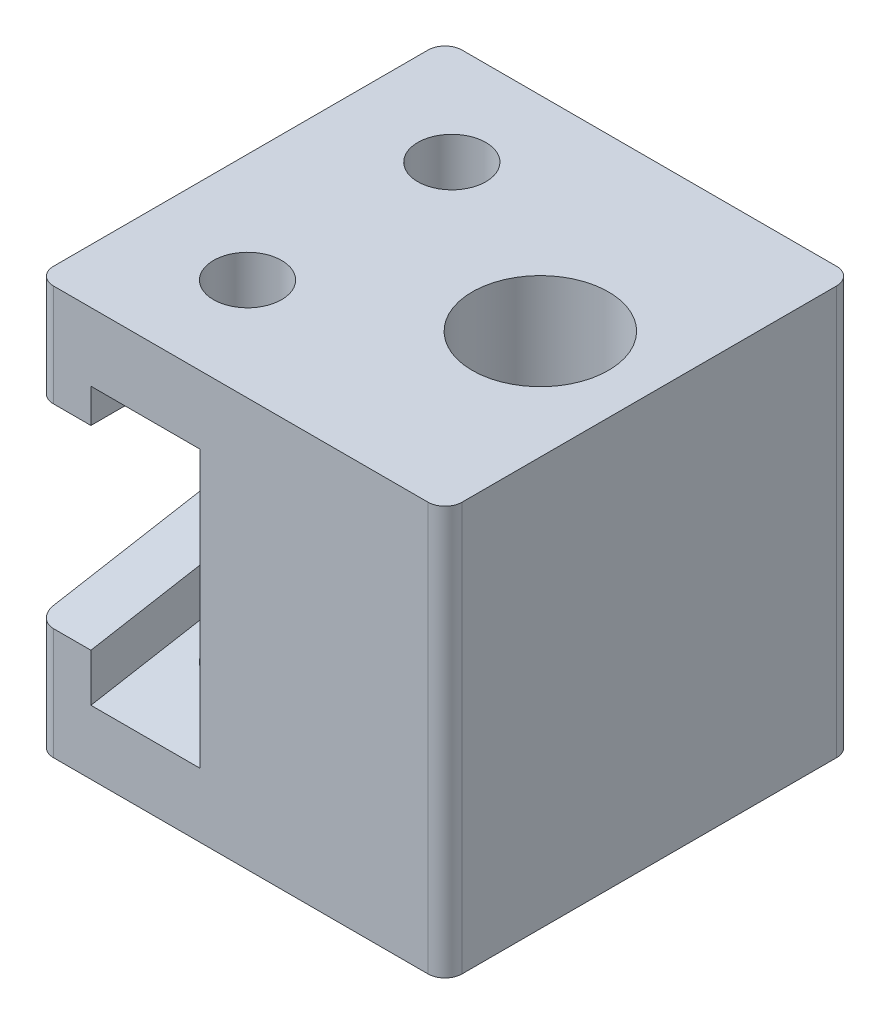
ISO-10303-21;
HEADER;
FILE_DESCRIPTION(('STEP AP214'),'2;1');
FILE_NAME('part.step','',(''),(''),'','','');
FILE_SCHEMA(('AUTOMOTIVE_DESIGN { 1 0 10303 214 1 1 1 1 }'));
ENDSEC;
DATA;
#1=APPLICATION_CONTEXT('core data for automotive mechanical design processes');
#2=APPLICATION_PROTOCOL_DEFINITION('international standard','automotive_design',2000,#1);
#3=PRODUCT_CONTEXT('',#1,'mechanical');
#4=PRODUCT('Part','Part','',(#3));
#5=PRODUCT_RELATED_PRODUCT_CATEGORY('part','',(#4));
#6=PRODUCT_DEFINITION_FORMATION('','',#4);
#7=PRODUCT_DEFINITION_CONTEXT('part definition',#1,'design');
#8=PRODUCT_DEFINITION('design','',#6,#7);
#9=PRODUCT_DEFINITION_SHAPE('','',#8);
#10=(LENGTH_UNIT() NAMED_UNIT(*) SI_UNIT(.MILLI.,.METRE.));
#11=(NAMED_UNIT(*) PLANE_ANGLE_UNIT() SI_UNIT($,.RADIAN.));
#12=(NAMED_UNIT(*) SI_UNIT($,.STERADIAN.) SOLID_ANGLE_UNIT());
#13=UNCERTAINTY_MEASURE_WITH_UNIT(LENGTH_MEASURE(1.E-05),#10,'distance_accuracy_value','');
#14=(GEOMETRIC_REPRESENTATION_CONTEXT(3) GLOBAL_UNCERTAINTY_ASSIGNED_CONTEXT((#13)) GLOBAL_UNIT_ASSIGNED_CONTEXT((#10,
#11,#12)) REPRESENTATION_CONTEXT('',''));
#15=CARTESIAN_POINT('',(0.,0.,0.));
#16=DIRECTION('',(0.,0.,1.));
#17=DIRECTION('',(1.,0.,0.));
#18=AXIS2_PLACEMENT_3D('',#15,#16,#17);
#19=CARTESIAN_POINT('',(0.,0.,38.1));
#20=DIRECTION('',(0.,0.,-1.));
#21=DIRECTION('',(-1.,0.,0.));
#22=AXIS2_PLACEMENT_3D('',#19,#20,#21);
#23=PLANE('',#22);
#24=DIRECTION('',(1.,0.,0.));
#25=VECTOR('',#24,1.);
#26=CARTESIAN_POINT('',(-38.1,-38.1,38.1));
#27=LINE('',#26,#25);
#28=CARTESIAN_POINT('',(-34.925,-38.1,38.1));
#29=VERTEX_POINT('',#28);
#30=CARTESIAN_POINT('',(34.925,-38.1,38.1));
#31=VERTEX_POINT('',#30);
#32=EDGE_CURVE('E229',#29,#31,#27,.T.);
#33=ORIENTED_EDGE('',*,*,#32,.T.);
#34=DIRECTION('',(0.,1.,0.));
#35=VECTOR('',#34,1.);
#36=CARTESIAN_POINT('',(34.925,0.,38.1));
#37=LINE('',#36,#35);
#38=CARTESIAN_POINT('',(34.925,38.1,38.1));
#39=VERTEX_POINT('',#38);
#40=EDGE_CURVE('E11',#31,#39,#37,.T.);
#41=ORIENTED_EDGE('',*,*,#40,.T.);
#42=DIRECTION('',(-1.,0.,0.));
#43=VECTOR('',#42,1.);
#44=CARTESIAN_POINT('',(-38.1,38.1,38.1));
#45=LINE('',#44,#43);
#46=CARTESIAN_POINT('',(-34.925,38.1,38.1));
#47=VERTEX_POINT('',#46);
#48=EDGE_CURVE('E223',#39,#47,#45,.T.);
#49=ORIENTED_EDGE('',*,*,#48,.T.);
#50=DIRECTION('',(0.,-1.,0.));
#51=VECTOR('',#50,1.);
#52=CARTESIAN_POINT('',(-34.925,0.,38.1));
#53=LINE('',#52,#51);
#54=CARTESIAN_POINT('',(-34.925,19.05,38.1));
#55=VERTEX_POINT('',#54);
#56=EDGE_CURVE('E289',#47,#55,#53,.T.);
#57=ORIENTED_EDGE('',*,*,#56,.T.);
#58=DIRECTION('',(-1.,0.,0.));
#59=VECTOR('',#58,1.);
#60=CARTESIAN_POINT('',(-27.94,19.05,38.1));
#61=LINE('',#60,#59);
#62=CARTESIAN_POINT('',(-27.94,19.05,38.1));
#63=VERTEX_POINT('',#62);
#64=EDGE_CURVE('E206',#63,#55,#61,.T.);
#65=ORIENTED_EDGE('',*,*,#64,.F.);
#66=DIRECTION('',(0.,1.,0.));
#67=VECTOR('',#66,1.);
#68=CARTESIAN_POINT('',(-27.94,25.4,38.1));
#69=LINE('',#68,#67);
#70=CARTESIAN_POINT('',(-27.94,25.4,38.1));
#71=VERTEX_POINT('',#70);
#72=EDGE_CURVE('E325',#63,#71,#69,.T.);
#73=ORIENTED_EDGE('',*,*,#72,.T.);
#74=DIRECTION('',(-1.,0.,0.));
#75=VECTOR('',#74,1.);
#76=CARTESIAN_POINT('',(-7.61999999999999,25.4,38.1));
#77=LINE('',#76,#75);
#78=CARTESIAN_POINT('',(-7.61999999999999,25.4,38.1));
#79=VERTEX_POINT('',#78);
#80=EDGE_CURVE('E198',#79,#71,#77,.T.);
#81=ORIENTED_EDGE('',*,*,#80,.F.);
#82=DIRECTION('',(0.,1.,0.));
#83=VECTOR('',#82,1.);
#84=CARTESIAN_POINT('',(-7.61999999999999,25.4,38.1));
#85=LINE('',#84,#83);
#86=CARTESIAN_POINT('',(-7.61999999999999,-26.1361159299851,38.1));
#87=VERTEX_POINT('',#86);
#88=EDGE_CURVE('E176',#87,#79,#85,.T.);
#89=ORIENTED_EDGE('',*,*,#88,.F.);
#90=DIRECTION('',(-1.,0.,0.));
#91=VECTOR('',#90,1.);
#92=CARTESIAN_POINT('',(-7.61999999999999,-26.1361159299851,38.1));
#93=LINE('',#92,#91);
#94=CARTESIAN_POINT('',(-27.94,-26.1361159299851,38.1));
#95=VERTEX_POINT('',#94);
#96=EDGE_CURVE('E175',#87,#95,#93,.T.);
#97=ORIENTED_EDGE('',*,*,#96,.T.);
#98=CARTESIAN_POINT('',(-27.94,-17.2461159299851,38.1));
#99=VERTEX_POINT('',#98);
#100=EDGE_CURVE('E323',#95,#99,#69,.T.);
#101=ORIENTED_EDGE('',*,*,#100,.T.);
#102=DIRECTION('',(-1.,0.,0.));
#103=VECTOR('',#102,1.);
#104=CARTESIAN_POINT('',(-27.94,-17.2461159299851,38.1));
#105=LINE('',#104,#103);
#106=CARTESIAN_POINT('',(-34.925,-17.2461159299851,38.1));
#107=VERTEX_POINT('',#106);
#108=EDGE_CURVE('E213',#99,#107,#105,.T.);
#109=ORIENTED_EDGE('',*,*,#108,.T.);
#110=DIRECTION('',(0.,-1.,0.));
#111=VECTOR('',#110,1.);
#112=CARTESIAN_POINT('',(-34.925,0.,38.1));
#113=LINE('',#112,#111);
#114=EDGE_CURVE('E48',#107,#29,#113,.T.);
#115=ORIENTED_EDGE('',*,*,#114,.T.);
#116=EDGE_LOOP('',(#33,#41,#49,#57,#65,#73,#81,#89,#97,#101,#109,#115));
#117=FACE_BOUND('',#116,.T.);
#118=ADVANCED_FACE('F39',(#117),#23,.F.);
#119=CARTESIAN_POINT('',(0.,0.,-38.1));
#120=DIRECTION('',(0.,0.,-1.));
#121=DIRECTION('',(-1.,0.,0.));
#122=AXIS2_PLACEMENT_3D('',#119,#120,#121);
#123=PLANE('',#122);
#124=DIRECTION('',(-1.,0.,0.));
#125=VECTOR('',#124,1.);
#126=CARTESIAN_POINT('',(-38.1,38.1,-38.1));
#127=LINE('',#126,#125);
#128=CARTESIAN_POINT('',(34.925,38.1,-38.1));
#129=VERTEX_POINT('',#128);
#130=CARTESIAN_POINT('',(-34.925,38.1,-38.1));
#131=VERTEX_POINT('',#130);
#132=EDGE_CURVE('E216',#129,#131,#127,.T.);
#133=ORIENTED_EDGE('',*,*,#132,.F.);
#134=DIRECTION('',(0.,1.,0.));
#135=VECTOR('',#134,1.);
#136=CARTESIAN_POINT('',(34.925,-38.1,-38.1));
#137=LINE('',#136,#135);
#138=CARTESIAN_POINT('',(34.925,-38.1,-38.1));
#139=VERTEX_POINT('',#138);
#140=EDGE_CURVE('E264',#129,#139,#137,.F.);
#141=ORIENTED_EDGE('',*,*,#140,.T.);
#142=DIRECTION('',(1.,0.,0.));
#143=VECTOR('',#142,1.);
#144=CARTESIAN_POINT('',(-38.1,-38.1,-38.1));
#145=LINE('',#144,#143);
#146=CARTESIAN_POINT('',(-34.925,-38.1,-38.1));
#147=VERTEX_POINT('',#146);
#148=EDGE_CURVE('E228',#147,#139,#145,.T.);
#149=ORIENTED_EDGE('',*,*,#148,.F.);
#150=DIRECTION('',(0.,-1.,0.));
#151=VECTOR('',#150,1.);
#152=CARTESIAN_POINT('',(-34.925,-3.80999999999999,-38.1));
#153=LINE('',#152,#151);
#154=CARTESIAN_POINT('',(-34.925,-3.80999999999999,-38.1));
#155=VERTEX_POINT('',#154);
#156=EDGE_CURVE('E263',#147,#155,#153,.F.);
#157=ORIENTED_EDGE('',*,*,#156,.T.);
#158=DIRECTION('',(-1.,0.,0.));
#159=VECTOR('',#158,1.);
#160=CARTESIAN_POINT('',(-27.94,-3.80999999999999,-38.1));
#161=LINE('',#160,#159);
#162=CARTESIAN_POINT('',(-27.94,-3.80999999999999,-38.1));
#163=VERTEX_POINT('',#162);
#164=EDGE_CURVE('E220',#163,#155,#161,.T.);
#165=ORIENTED_EDGE('',*,*,#164,.F.);
#166=DIRECTION('',(0.,-1.,0.));
#167=VECTOR('',#166,1.);
#168=CARTESIAN_POINT('',(-27.94,-12.6999999999997,-38.1));
#169=LINE('',#168,#167);
#170=CARTESIAN_POINT('',(-27.94,-12.6999999999997,-38.1));
#171=VERTEX_POINT('',#170);
#172=EDGE_CURVE('E192',#163,#171,#169,.T.);
#173=ORIENTED_EDGE('',*,*,#172,.T.);
#174=DIRECTION('',(-1.,0.,0.));
#175=VECTOR('',#174,1.);
#176=CARTESIAN_POINT('',(-7.61999999999999,-12.6999999999997,-38.1));
#177=LINE('',#176,#175);
#178=CARTESIAN_POINT('',(-7.61999999999999,-12.6999999999997,-38.1));
#179=VERTEX_POINT('',#178);
#180=EDGE_CURVE('E172',#179,#171,#177,.T.);
#181=ORIENTED_EDGE('',*,*,#180,.F.);
#182=DIRECTION('',(0.,-1.,0.));
#183=VECTOR('',#182,1.);
#184=CARTESIAN_POINT('',(-7.61999999999999,-12.6999999999997,-38.1));
#185=LINE('',#184,#183);
#186=CARTESIAN_POINT('',(-7.61999999999999,25.4,-38.1));
#187=VERTEX_POINT('',#186);
#188=EDGE_CURVE('E177',#187,#179,#185,.T.);
#189=ORIENTED_EDGE('',*,*,#188,.F.);
#190=DIRECTION('',(-1.,0.,0.));
#191=VECTOR('',#190,1.);
#192=CARTESIAN_POINT('',(-7.61999999999999,25.4,-38.1));
#193=LINE('',#192,#191);
#194=CARTESIAN_POINT('',(-27.94,25.4,-38.1));
#195=VERTEX_POINT('',#194);
#196=EDGE_CURVE('E209',#187,#195,#193,.T.);
#197=ORIENTED_EDGE('',*,*,#196,.T.);
#198=CARTESIAN_POINT('',(-27.94,19.05,-38.1));
#199=VERTEX_POINT('',#198);
#200=EDGE_CURVE('E320',#195,#199,#169,.T.);
#201=ORIENTED_EDGE('',*,*,#200,.T.);
#202=DIRECTION('',(-1.,0.,0.));
#203=VECTOR('',#202,1.);
#204=CARTESIAN_POINT('',(-27.94,19.05,-38.1));
#205=LINE('',#204,#203);
#206=CARTESIAN_POINT('',(-34.925,19.05,-38.1));
#207=VERTEX_POINT('',#206);
#208=EDGE_CURVE('E219',#199,#207,#205,.T.);
#209=ORIENTED_EDGE('',*,*,#208,.T.);
#210=DIRECTION('',(0.,-1.,0.));
#211=VECTOR('',#210,1.);
#212=CARTESIAN_POINT('',(-34.925,38.1,-38.1));
#213=LINE('',#212,#211);
#214=EDGE_CURVE('E261',#207,#131,#213,.F.);
#215=ORIENTED_EDGE('',*,*,#214,.T.);
#216=EDGE_LOOP('',(#133,#141,#149,#157,#165,#173,#181,#189,#197,#201,#209,#215));
#217=FACE_BOUND('',#216,.T.);
#218=ADVANCED_FACE('F195',(#217),#123,.T.);
#219=CARTESIAN_POINT('',(-38.1,-38.1,38.1));
#220=DIRECTION('',(1.,0.,0.));
#221=DIRECTION('',(0.,0.,-1.));
#222=AXIS2_PLACEMENT_3D('',#219,#220,#221);
#223=PLANE('',#222);
#224=DIRECTION('',(0.,-0.173648177666931,0.984807753012208));
#225=VECTOR('',#224,1.);
#226=CARTESIAN_POINT('',(-38.1,-17.2461159299851,38.1));
#227=LINE('',#226,#225);
#228=CARTESIAN_POINT('',(-38.1,-4.36983816374937,-34.925));
#229=VERTEX_POINT('',#228);
#230=CARTESIAN_POINT('',(-38.1,-16.6862777662357,34.925));
#231=VERTEX_POINT('',#230);
#232=EDGE_CURVE('E204',#229,#231,#227,.T.);
#233=ORIENTED_EDGE('',*,*,#232,.F.);
#234=DIRECTION('',(0.,-1.,0.));
#235=VECTOR('',#234,1.);
#236=CARTESIAN_POINT('',(-38.1,-38.1,-34.925));
#237=LINE('',#236,#235);
#238=CARTESIAN_POINT('',(-38.1,-38.1,-34.925));
#239=VERTEX_POINT('',#238);
#240=EDGE_CURVE('E280',#229,#239,#237,.T.);
#241=ORIENTED_EDGE('',*,*,#240,.T.);
#242=DIRECTION('',(0.,0.,-1.));
#243=VECTOR('',#242,1.);
#244=CARTESIAN_POINT('',(-38.1,-38.1,38.1));
#245=LINE('',#244,#243);
#246=CARTESIAN_POINT('',(-38.1,-38.1,34.925));
#247=VERTEX_POINT('',#246);
#248=EDGE_CURVE('E239',#247,#239,#245,.T.);
#249=ORIENTED_EDGE('',*,*,#248,.F.);
#250=DIRECTION('',(0.,-1.,0.));
#251=VECTOR('',#250,1.);
#252=CARTESIAN_POINT('',(-38.1,-38.1,34.925));
#253=LINE('',#252,#251);
#254=EDGE_CURVE('E274',#247,#231,#253,.F.);
#255=ORIENTED_EDGE('',*,*,#254,.T.);
#256=EDGE_LOOP('',(#233,#241,#249,#255));
#257=FACE_BOUND('',#256,.T.);
#258=ADVANCED_FACE('F380',(#257),#223,.F.);
#259=CARTESIAN_POINT('',(38.1,-38.1,38.1));
#260=DIRECTION('',(-1.,0.,0.));
#261=DIRECTION('',(0.,0.,1.));
#262=AXIS2_PLACEMENT_3D('',#259,#260,#261);
#263=PLANE('',#262);
#264=DIRECTION('',(0.,0.,-1.));
#265=VECTOR('',#264,1.);
#266=CARTESIAN_POINT('',(38.1,-38.1,38.1));
#267=LINE('',#266,#265);
#268=CARTESIAN_POINT('',(38.1,-38.1,34.925));
#269=VERTEX_POINT('',#268);
#270=CARTESIAN_POINT('',(38.1,-38.1,-34.925));
#271=VERTEX_POINT('',#270);
#272=EDGE_CURVE('E235',#269,#271,#267,.T.);
#273=ORIENTED_EDGE('',*,*,#272,.T.);
#274=DIRECTION('',(0.,1.,0.));
#275=VECTOR('',#274,1.);
#276=CARTESIAN_POINT('',(38.1,38.1,-34.925));
#277=LINE('',#276,#275);
#278=CARTESIAN_POINT('',(38.1,38.1,-34.925));
#279=VERTEX_POINT('',#278);
#280=EDGE_CURVE('E249',#271,#279,#277,.T.);
#281=ORIENTED_EDGE('',*,*,#280,.T.);
#282=DIRECTION('',(0.,0.,-1.));
#283=VECTOR('',#282,1.);
#284=CARTESIAN_POINT('',(38.1,38.1,38.1));
#285=LINE('',#284,#283);
#286=CARTESIAN_POINT('',(38.1,38.1,34.925));
#287=VERTEX_POINT('',#286);
#288=EDGE_CURVE('E245',#287,#279,#285,.T.);
#289=ORIENTED_EDGE('',*,*,#288,.F.);
#290=DIRECTION('',(0.,1.,0.));
#291=VECTOR('',#290,1.);
#292=CARTESIAN_POINT('',(38.1,-38.1,34.925));
#293=LINE('',#292,#291);
#294=EDGE_CURVE('E246',#287,#269,#293,.F.);
#295=ORIENTED_EDGE('',*,*,#294,.T.);
#296=EDGE_LOOP('',(#273,#281,#289,#295));
#297=FACE_BOUND('',#296,.T.);
#298=ADVANCED_FACE('F357',(#297),#263,.F.);
#299=CARTESIAN_POINT('',(-38.1,38.1,38.1));
#300=DIRECTION('',(0.,-1.,0.));
#301=DIRECTION('',(0.,0.,-1.));
#302=AXIS2_PLACEMENT_3D('',#299,#300,#301);
#303=PLANE('',#302);
#304=CARTESIAN_POINT('',(17.78,38.1,0.));
#305=DIRECTION('',(0.,1.,0.));
#306=DIRECTION('',(0.,0.,1.));
#307=AXIS2_PLACEMENT_3D('',#304,#305,#306);
#308=CIRCLE('',#307,12.7);
#309=CARTESIAN_POINT('',(17.78,38.1,12.7));
#310=VERTEX_POINT('',#309);
#311=EDGE_CURVE('E309',#310,#310,#308,.T.);
#312=ORIENTED_EDGE('',*,*,#311,.F.);
#313=EDGE_LOOP('',(#312));
#314=FACE_BOUND('',#313,.T.);
#315=CARTESIAN_POINT('',(-17.78,38.1,19.05));
#316=DIRECTION('',(0.,1.,0.));
#317=DIRECTION('',(0.,0.,1.));
#318=AXIS2_PLACEMENT_3D('',#315,#316,#317);
#319=CIRCLE('',#318,6.35);
#320=CARTESIAN_POINT('',(-17.78,38.1,25.4));
#321=VERTEX_POINT('',#320);
#322=EDGE_CURVE('E541',#321,#321,#319,.T.);
#323=ORIENTED_EDGE('',*,*,#322,.F.);
#324=EDGE_LOOP('',(#323));
#325=FACE_BOUND('',#324,.T.);
#326=CARTESIAN_POINT('',(-17.78,38.1,-19.05));
#327=DIRECTION('',(0.,1.,0.));
#328=DIRECTION('',(0.,0.,1.));
#329=AXIS2_PLACEMENT_3D('',#326,#327,#328);
#330=CIRCLE('',#329,6.35);
#331=CARTESIAN_POINT('',(-17.78,38.1,-12.7));
#332=VERTEX_POINT('',#331);
#333=EDGE_CURVE('E305',#332,#332,#330,.T.);
#334=ORIENTED_EDGE('',*,*,#333,.F.);
#335=EDGE_LOOP('',(#334));
#336=FACE_BOUND('',#335,.T.);
#337=ORIENTED_EDGE('',*,*,#288,.T.);
#338=CARTESIAN_POINT('',(34.925,38.1,-34.925));
#339=DIRECTION('',(0.,-1.,0.));
#340=DIRECTION('',(0.,0.,-1.));
#341=AXIS2_PLACEMENT_3D('',#338,#339,#340);
#342=CIRCLE('',#341,3.175);
#343=EDGE_CURVE('E259',#279,#129,#342,.F.);
#344=ORIENTED_EDGE('',*,*,#343,.T.);
#345=ORIENTED_EDGE('',*,*,#132,.T.);
#346=CARTESIAN_POINT('',(-34.925,38.1,-34.925));
#347=DIRECTION('',(0.,-1.,0.));
#348=DIRECTION('',(0.,0.,-1.));
#349=AXIS2_PLACEMENT_3D('',#346,#347,#348);
#350=CIRCLE('',#349,3.175);
#351=CARTESIAN_POINT('',(-38.1,38.1,-34.925));
#352=VERTEX_POINT('',#351);
#353=EDGE_CURVE('E260',#131,#352,#350,.F.);
#354=ORIENTED_EDGE('',*,*,#353,.T.);
#355=DIRECTION('',(0.,0.,-1.));
#356=VECTOR('',#355,1.);
#357=CARTESIAN_POINT('',(-38.1,38.1,38.1));
#358=LINE('',#357,#356);
#359=CARTESIAN_POINT('',(-38.1,38.1,34.925));
#360=VERTEX_POINT('',#359);
#361=EDGE_CURVE('E242',#360,#352,#358,.T.);
#362=ORIENTED_EDGE('',*,*,#361,.F.);
#363=CARTESIAN_POINT('',(-34.925,38.1,34.925));
#364=DIRECTION('',(0.,-1.,0.));
#365=DIRECTION('',(0.,0.,-1.));
#366=AXIS2_PLACEMENT_3D('',#363,#364,#365);
#367=CIRCLE('',#366,3.175);
#368=EDGE_CURVE('E251',#360,#47,#367,.F.);
#369=ORIENTED_EDGE('',*,*,#368,.T.);
#370=ORIENTED_EDGE('',*,*,#48,.F.);
#371=CARTESIAN_POINT('',(34.925,38.1,34.925));
#372=DIRECTION('',(0.,-1.,0.));
#373=DIRECTION('',(0.,0.,-1.));
#374=AXIS2_PLACEMENT_3D('',#371,#372,#373);
#375=CIRCLE('',#374,3.175);
#376=EDGE_CURVE('E254',#39,#287,#375,.F.);
#377=ORIENTED_EDGE('',*,*,#376,.T.);
#378=EDGE_LOOP('',(#337,#344,#345,#354,#362,#369,#370,#377));
#379=FACE_BOUND('',#378,.T.);
#380=ADVANCED_FACE('F347',(#314,#325,#336,#379),#303,.F.);
#381=ORIENTED_EDGE('',*,*,#361,.T.);
#382=DIRECTION('',(0.,-1.,0.));
#383=VECTOR('',#382,1.);
#384=CARTESIAN_POINT('',(-38.1,19.05,-34.925));
#385=LINE('',#384,#383);
#386=CARTESIAN_POINT('',(-38.1,19.05,-34.925));
#387=VERTEX_POINT('',#386);
#388=EDGE_CURVE('E288',#352,#387,#385,.T.);
#389=ORIENTED_EDGE('',*,*,#388,.T.);
#390=DIRECTION('',(0.,0.,-1.));
#391=VECTOR('',#390,1.);
#392=CARTESIAN_POINT('',(-38.1,19.05,-38.1));
#393=LINE('',#392,#391);
#394=CARTESIAN_POINT('',(-38.1,19.05,34.925));
#395=VERTEX_POINT('',#394);
#396=EDGE_CURVE('E210',#395,#387,#393,.T.);
#397=ORIENTED_EDGE('',*,*,#396,.F.);
#398=DIRECTION('',(0.,-1.,0.));
#399=VECTOR('',#398,1.);
#400=CARTESIAN_POINT('',(-38.1,-38.1,34.925));
#401=LINE('',#400,#399);
#402=EDGE_CURVE('E283',#395,#360,#401,.F.);
#403=ORIENTED_EDGE('',*,*,#402,.T.);
#404=EDGE_LOOP('',(#381,#389,#397,#403));
#405=FACE_BOUND('',#404,.T.);
#406=ADVANCED_FACE('F349',(#405),#223,.F.);
#407=CARTESIAN_POINT('',(-38.1,-38.1,38.1));
#408=DIRECTION('',(0.,1.,0.));
#409=DIRECTION('',(0.,0.,1.));
#410=AXIS2_PLACEMENT_3D('',#407,#408,#409);
#411=PLANE('',#410);
#412=CARTESIAN_POINT('',(17.78,-38.1,0.));
#413=DIRECTION('',(0.,1.,0.));
#414=DIRECTION('',(0.,0.,1.));
#415=AXIS2_PLACEMENT_3D('',#412,#413,#414);
#416=CIRCLE('',#415,12.7);
#417=CARTESIAN_POINT('',(17.78,-38.1,12.7));
#418=VERTEX_POINT('',#417);
#419=EDGE_CURVE('E538',#418,#418,#416,.T.);
#420=ORIENTED_EDGE('',*,*,#419,.T.);
#421=EDGE_LOOP('',(#420));
#422=FACE_BOUND('',#421,.T.);
#423=CARTESIAN_POINT('',(-17.78,-38.1,19.05));
#424=DIRECTION('',(0.,1.,0.));
#425=DIRECTION('',(0.,0.,1.));
#426=AXIS2_PLACEMENT_3D('',#423,#424,#425);
#427=CIRCLE('',#426,6.35);
#428=CARTESIAN_POINT('',(-17.78,-38.1,25.4));
#429=VERTEX_POINT('',#428);
#430=EDGE_CURVE('E307',#429,#429,#427,.T.);
#431=ORIENTED_EDGE('',*,*,#430,.T.);
#432=EDGE_LOOP('',(#431));
#433=FACE_BOUND('',#432,.T.);
#434=CARTESIAN_POINT('',(-17.78,-38.1,-19.05));
#435=DIRECTION('',(0.,1.,0.));
#436=DIRECTION('',(0.,0.,1.));
#437=AXIS2_PLACEMENT_3D('',#434,#435,#436);
#438=CIRCLE('',#437,6.35);
#439=CARTESIAN_POINT('',(-17.78,-38.1,-12.7));
#440=VERTEX_POINT('',#439);
#441=EDGE_CURVE('E296',#440,#440,#438,.T.);
#442=ORIENTED_EDGE('',*,*,#441,.T.);
#443=EDGE_LOOP('',(#442));
#444=FACE_BOUND('',#443,.T.);
#445=ORIENTED_EDGE('',*,*,#148,.T.);
#446=CARTESIAN_POINT('',(34.925,-38.1,-34.925));
#447=DIRECTION('',(0.,1.,0.));
#448=DIRECTION('',(0.,0.,1.));
#449=AXIS2_PLACEMENT_3D('',#446,#447,#448);
#450=CIRCLE('',#449,3.175);
#451=EDGE_CURVE('E272',#139,#271,#450,.F.);
#452=ORIENTED_EDGE('',*,*,#451,.T.);
#453=ORIENTED_EDGE('',*,*,#272,.F.);
#454=CARTESIAN_POINT('',(34.925,-38.1,34.925));
#455=DIRECTION('',(0.,1.,0.));
#456=DIRECTION('',(0.,0.,1.));
#457=AXIS2_PLACEMENT_3D('',#454,#455,#456);
#458=CIRCLE('',#457,3.175);
#459=EDGE_CURVE('E267',#269,#31,#458,.F.);
#460=ORIENTED_EDGE('',*,*,#459,.T.);
#461=ORIENTED_EDGE('',*,*,#32,.F.);
#462=CARTESIAN_POINT('',(-34.925,-38.1,34.925));
#463=DIRECTION('',(0.,1.,0.));
#464=DIRECTION('',(0.,0.,1.));
#465=AXIS2_PLACEMENT_3D('',#462,#463,#464);
#466=CIRCLE('',#465,3.175);
#467=EDGE_CURVE('E270',#29,#247,#466,.F.);
#468=ORIENTED_EDGE('',*,*,#467,.T.);
#469=ORIENTED_EDGE('',*,*,#248,.T.);
#470=CARTESIAN_POINT('',(-34.925,-38.1,-34.925));
#471=DIRECTION('',(0.,1.,0.));
#472=DIRECTION('',(0.,0.,1.));
#473=AXIS2_PLACEMENT_3D('',#470,#471,#472);
#474=CIRCLE('',#473,3.175);
#475=EDGE_CURVE('E271',#239,#147,#474,.F.);
#476=ORIENTED_EDGE('',*,*,#475,.T.);
#477=EDGE_LOOP('',(#445,#452,#453,#460,#461,#468,#469,#476));
#478=FACE_BOUND('',#477,.T.);
#479=ADVANCED_FACE('F369',(#422,#433,#444,#478),#411,.F.);
#480=CARTESIAN_POINT('',(-27.94,-17.2461159299851,38.1));
#481=DIRECTION('',(0.,-0.984807753012208,-0.173648177666931));
#482=DIRECTION('',(0.,0.173648177666931,-0.984807753012208));
#483=AXIS2_PLACEMENT_3D('',#480,#481,#482);
#484=PLANE('',#483);
#485=ORIENTED_EDGE('',*,*,#164,.T.);
#486=CARTESIAN_POINT('',(-34.925,-4.36983816374937,-34.925));
#487=DIRECTION('',(0.,-0.984807753012208,-0.173648177666931));
#488=DIRECTION('',(0.,0.173648177666931,-0.984807753012208));
#489=AXIS2_PLACEMENT_3D('',#486,#487,#488);
#490=ELLIPSE('',#489,3.22397949273724,3.175);
#491=EDGE_CURVE('E282',#155,#229,#490,.F.);
#492=ORIENTED_EDGE('',*,*,#491,.T.);
#493=ORIENTED_EDGE('',*,*,#232,.T.);
#494=CARTESIAN_POINT('',(-34.925,-16.6862777662357,34.925));
#495=DIRECTION('',(0.,-0.984807753012208,-0.173648177666931));
#496=DIRECTION('',(0.,-0.173648177666931,0.984807753012208));
#497=AXIS2_PLACEMENT_3D('',#494,#495,#496);
#498=ELLIPSE('',#497,3.22397949273724,3.175);
#499=EDGE_CURVE('E278',#231,#107,#498,.F.);
#500=ORIENTED_EDGE('',*,*,#499,.T.);
#501=ORIENTED_EDGE('',*,*,#108,.F.);
#502=DIRECTION('',(0.,-0.173648177666931,0.984807753012208));
#503=VECTOR('',#502,1.);
#504=CARTESIAN_POINT('',(-27.94,-17.2461159299851,38.1));
#505=LINE('',#504,#503);
#506=EDGE_CURVE('E201',#163,#99,#505,.T.);
#507=ORIENTED_EDGE('',*,*,#506,.F.);
#508=EDGE_LOOP('',(#485,#492,#493,#500,#501,#507));
#509=FACE_BOUND('',#508,.T.);
#510=ADVANCED_FACE('F381',(#509),#484,.F.);
#511=CARTESIAN_POINT('',(-27.94,19.05,-38.1));
#512=DIRECTION('',(0.,1.,0.));
#513=DIRECTION('',(0.,0.,1.));
#514=AXIS2_PLACEMENT_3D('',#511,#512,#513);
#515=PLANE('',#514);
#516=ORIENTED_EDGE('',*,*,#396,.T.);
#517=CARTESIAN_POINT('',(-34.925,19.05,-34.925));
#518=DIRECTION('',(0.,1.,0.));
#519=DIRECTION('',(0.,0.,1.));
#520=AXIS2_PLACEMENT_3D('',#517,#518,#519);
#521=CIRCLE('',#520,3.175);
#522=EDGE_CURVE('E63',#387,#207,#521,.F.);
#523=ORIENTED_EDGE('',*,*,#522,.T.);
#524=ORIENTED_EDGE('',*,*,#208,.F.);
#525=DIRECTION('',(0.,0.,-1.));
#526=VECTOR('',#525,1.);
#527=CARTESIAN_POINT('',(-27.94,19.05,-38.1));
#528=LINE('',#527,#526);
#529=EDGE_CURVE('E203',#63,#199,#528,.T.);
#530=ORIENTED_EDGE('',*,*,#529,.F.);
#531=ORIENTED_EDGE('',*,*,#64,.T.);
#532=CARTESIAN_POINT('',(-34.925,19.05,34.925));
#533=DIRECTION('',(0.,1.,0.));
#534=DIRECTION('',(0.,0.,1.));
#535=AXIS2_PLACEMENT_3D('',#532,#533,#534);
#536=CIRCLE('',#535,3.175);
#537=EDGE_CURVE('E57',#55,#395,#536,.F.);
#538=ORIENTED_EDGE('',*,*,#537,.T.);
#539=EDGE_LOOP('',(#516,#523,#524,#530,#531,#538));
#540=FACE_BOUND('',#539,.T.);
#541=ADVANCED_FACE('F338',(#540),#515,.F.);
#542=CARTESIAN_POINT('',(-27.94,0.,0.));
#543=DIRECTION('',(1.,0.,0.));
#544=DIRECTION('',(0.,0.,-1.));
#545=AXIS2_PLACEMENT_3D('',#542,#543,#544);
#546=PLANE('',#545);
#547=ORIENTED_EDGE('',*,*,#506,.T.);
#548=ORIENTED_EDGE('',*,*,#100,.F.);
#549=DIRECTION('',(0.,-0.173648177666934,0.984807753012207));
#550=VECTOR('',#549,1.);
#551=CARTESIAN_POINT('',(-27.94,-26.1361159299851,38.1));
#552=LINE('',#551,#550);
#553=EDGE_CURVE('E319',#171,#95,#552,.T.);
#554=ORIENTED_EDGE('',*,*,#553,.F.);
#555=ORIENTED_EDGE('',*,*,#172,.F.);
#556=EDGE_LOOP('',(#547,#548,#554,#555));
#557=FACE_BOUND('',#556,.T.);
#558=ADVANCED_FACE('F389',(#557),#546,.T.);
#559=ORIENTED_EDGE('',*,*,#529,.T.);
#560=ORIENTED_EDGE('',*,*,#200,.F.);
#561=DIRECTION('',(0.,0.,-1.));
#562=VECTOR('',#561,1.);
#563=CARTESIAN_POINT('',(-27.94,25.4,-38.1));
#564=LINE('',#563,#562);
#565=EDGE_CURVE('E189',#71,#195,#564,.T.);
#566=ORIENTED_EDGE('',*,*,#565,.F.);
#567=ORIENTED_EDGE('',*,*,#72,.F.);
#568=EDGE_LOOP('',(#559,#560,#566,#567));
#569=FACE_BOUND('',#568,.T.);
#570=ADVANCED_FACE('F333',(#569),#546,.T.);
#571=CARTESIAN_POINT('',(-7.61999999999999,25.4,-38.1));
#572=DIRECTION('',(0.,1.,0.));
#573=DIRECTION('',(0.,0.,1.));
#574=AXIS2_PLACEMENT_3D('',#571,#572,#573);
#575=PLANE('',#574);
#576=CARTESIAN_POINT('',(-17.78,25.4,19.05));
#577=DIRECTION('',(0.,1.,0.));
#578=DIRECTION('',(0.,0.,1.));
#579=AXIS2_PLACEMENT_3D('',#576,#577,#578);
#580=CIRCLE('',#579,6.35);
#581=CARTESIAN_POINT('',(-17.78,25.4,25.4));
#582=VERTEX_POINT('',#581);
#583=EDGE_CURVE('E311',#582,#582,#580,.T.);
#584=ORIENTED_EDGE('',*,*,#583,.T.);
#585=EDGE_LOOP('',(#584));
#586=FACE_BOUND('',#585,.T.);
#587=CARTESIAN_POINT('',(-17.78,25.4,-19.05));
#588=DIRECTION('',(0.,1.,0.));
#589=DIRECTION('',(0.,0.,1.));
#590=AXIS2_PLACEMENT_3D('',#587,#588,#589);
#591=CIRCLE('',#590,6.35);
#592=CARTESIAN_POINT('',(-17.78,25.4,-12.7));
#593=VERTEX_POINT('',#592);
#594=EDGE_CURVE('E293',#593,#593,#591,.T.);
#595=ORIENTED_EDGE('',*,*,#594,.T.);
#596=EDGE_LOOP('',(#595));
#597=FACE_BOUND('',#596,.T.);
#598=ORIENTED_EDGE('',*,*,#565,.T.);
#599=ORIENTED_EDGE('',*,*,#196,.F.);
#600=DIRECTION('',(0.,0.,-1.));
#601=VECTOR('',#600,1.);
#602=CARTESIAN_POINT('',(-7.61999999999999,25.4,-38.1));
#603=LINE('',#602,#601);
#604=EDGE_CURVE('E183',#79,#187,#603,.T.);
#605=ORIENTED_EDGE('',*,*,#604,.F.);
#606=ORIENTED_EDGE('',*,*,#80,.T.);
#607=EDGE_LOOP('',(#598,#599,#605,#606));
#608=FACE_BOUND('',#607,.T.);
#609=ADVANCED_FACE('F332',(#586,#597,#608),#575,.F.);
#610=CARTESIAN_POINT('',(-7.61999999999999,-26.1361159299851,38.1));
#611=DIRECTION('',(0.,-0.984807753012207,-0.173648177666934));
#612=DIRECTION('',(0.,0.173648177666934,-0.984807753012207));
#613=AXIS2_PLACEMENT_3D('',#610,#611,#612);
#614=PLANE('',#613);
#615=CARTESIAN_POINT('',(-17.78,-22.7770869474887,19.05));
#616=DIRECTION('',(0.,-0.984807753012207,-0.173648177666934));
#617=DIRECTION('',(0.,0.173648177666934,-0.984807753012207));
#618=AXIS2_PLACEMENT_3D('',#615,#616,#617);
#619=ELLIPSE('',#618,6.44795898547449,6.35);
#620=CARTESIAN_POINT('',(-17.78,-21.6574106199899,12.7));
#621=VERTEX_POINT('',#620);
#622=EDGE_CURVE('E43',#621,#621,#619,.T.);
#623=ORIENTED_EDGE('',*,*,#622,.T.);
#624=EDGE_LOOP('',(#623));
#625=FACE_BOUND('',#624,.T.);
#626=CARTESIAN_POINT('',(-17.78,-16.059028982496,-19.05));
#627=DIRECTION('',(0.,-0.984807753012207,-0.173648177666934));
#628=DIRECTION('',(0.,0.173648177666934,-0.984807753012207));
#629=AXIS2_PLACEMENT_3D('',#626,#627,#628);
#630=ELLIPSE('',#629,6.44795898547449,6.35);
#631=CARTESIAN_POINT('',(-17.78,-14.9393526549973,-25.4));
#632=VERTEX_POINT('',#631);
#633=EDGE_CURVE('E291',#632,#632,#630,.T.);
#634=ORIENTED_EDGE('',*,*,#633,.T.);
#635=EDGE_LOOP('',(#634));
#636=FACE_BOUND('',#635,.T.);
#637=ORIENTED_EDGE('',*,*,#553,.T.);
#638=ORIENTED_EDGE('',*,*,#96,.F.);
#639=DIRECTION('',(0.,-0.173648177666934,0.984807753012207));
#640=VECTOR('',#639,1.);
#641=CARTESIAN_POINT('',(-7.61999999999999,-26.1361159299851,38.1));
#642=LINE('',#641,#640);
#643=EDGE_CURVE('E170',#179,#87,#642,.T.);
#644=ORIENTED_EDGE('',*,*,#643,.F.);
#645=ORIENTED_EDGE('',*,*,#180,.T.);
#646=EDGE_LOOP('',(#637,#638,#644,#645));
#647=FACE_BOUND('',#646,.T.);
#648=ADVANCED_FACE('F168',(#625,#636,#647),#614,.F.);
#649=CARTESIAN_POINT('',(-7.61999999999999,0.,0.));
#650=DIRECTION('',(1.,0.,0.));
#651=DIRECTION('',(0.,0.,-1.));
#652=AXIS2_PLACEMENT_3D('',#649,#650,#651);
#653=PLANE('',#652);
#654=ORIENTED_EDGE('',*,*,#188,.T.);
#655=ORIENTED_EDGE('',*,*,#643,.T.);
#656=ORIENTED_EDGE('',*,*,#88,.T.);
#657=ORIENTED_EDGE('',*,*,#604,.T.);
#658=EDGE_LOOP('',(#654,#655,#656,#657));
#659=FACE_BOUND('',#658,.T.);
#660=ADVANCED_FACE('F181',(#659),#653,.F.);
#661=CARTESIAN_POINT('',(34.925,-38.1,-34.925));
#662=DIRECTION('',(0.,-1.,0.));
#663=DIRECTION('',(0.,0.,-1.));
#664=AXIS2_PLACEMENT_3D('',#661,#662,#663);
#665=CYLINDRICAL_SURFACE('',#664,3.175);
#666=ORIENTED_EDGE('',*,*,#451,.F.);
#667=ORIENTED_EDGE('',*,*,#140,.F.);
#668=ORIENTED_EDGE('',*,*,#343,.F.);
#669=ORIENTED_EDGE('',*,*,#280,.F.);
#670=EDGE_LOOP('',(#666,#667,#668,#669));
#671=FACE_BOUND('',#670,.T.);
#672=ADVANCED_FACE('F365',(#671),#665,.T.);
#673=CARTESIAN_POINT('',(-34.925,-38.1,-34.925));
#674=DIRECTION('',(0.,1.,0.));
#675=DIRECTION('',(0.,0.,1.));
#676=AXIS2_PLACEMENT_3D('',#673,#674,#675);
#677=CYLINDRICAL_SURFACE('',#676,3.175);
#678=ORIENTED_EDGE('',*,*,#491,.F.);
#679=ORIENTED_EDGE('',*,*,#156,.F.);
#680=ORIENTED_EDGE('',*,*,#475,.F.);
#681=ORIENTED_EDGE('',*,*,#240,.F.);
#682=EDGE_LOOP('',(#678,#679,#680,#681));
#683=FACE_BOUND('',#682,.T.);
#684=ADVANCED_FACE('F372',(#683),#677,.T.);
#685=CARTESIAN_POINT('',(-34.925,-38.1,-34.925));
#686=DIRECTION('',(0.,1.,0.));
#687=DIRECTION('',(0.,0.,1.));
#688=AXIS2_PLACEMENT_3D('',#685,#686,#687);
#689=CYLINDRICAL_SURFACE('',#688,3.175);
#690=ORIENTED_EDGE('',*,*,#353,.F.);
#691=ORIENTED_EDGE('',*,*,#214,.F.);
#692=ORIENTED_EDGE('',*,*,#522,.F.);
#693=ORIENTED_EDGE('',*,*,#388,.F.);
#694=EDGE_LOOP('',(#690,#691,#692,#693));
#695=FACE_BOUND('',#694,.T.);
#696=ADVANCED_FACE('F341',(#695),#689,.T.);
#697=CARTESIAN_POINT('',(34.925,0.,34.925));
#698=DIRECTION('',(0.,1.,0.));
#699=DIRECTION('',(0.,0.,1.));
#700=AXIS2_PLACEMENT_3D('',#697,#698,#699);
#701=CYLINDRICAL_SURFACE('',#700,3.175);
#702=ORIENTED_EDGE('',*,*,#459,.F.);
#703=ORIENTED_EDGE('',*,*,#294,.F.);
#704=ORIENTED_EDGE('',*,*,#376,.F.);
#705=ORIENTED_EDGE('',*,*,#40,.F.);
#706=EDGE_LOOP('',(#702,#703,#704,#705));
#707=FACE_BOUND('',#706,.T.);
#708=ADVANCED_FACE('F355',(#707),#701,.T.);
#709=CARTESIAN_POINT('',(-34.925,0.,34.925));
#710=DIRECTION('',(0.,-1.,0.));
#711=DIRECTION('',(0.,0.,-1.));
#712=AXIS2_PLACEMENT_3D('',#709,#710,#711);
#713=CYLINDRICAL_SURFACE('',#712,3.175);
#714=ORIENTED_EDGE('',*,*,#499,.F.);
#715=ORIENTED_EDGE('',*,*,#254,.F.);
#716=ORIENTED_EDGE('',*,*,#467,.F.);
#717=ORIENTED_EDGE('',*,*,#114,.F.);
#718=EDGE_LOOP('',(#714,#715,#716,#717));
#719=FACE_BOUND('',#718,.T.);
#720=ADVANCED_FACE('F384',(#719),#713,.T.);
#721=CARTESIAN_POINT('',(-34.925,0.,34.925));
#722=DIRECTION('',(0.,-1.,0.));
#723=DIRECTION('',(0.,0.,-1.));
#724=AXIS2_PLACEMENT_3D('',#721,#722,#723);
#725=CYLINDRICAL_SURFACE('',#724,3.175);
#726=ORIENTED_EDGE('',*,*,#368,.F.);
#727=ORIENTED_EDGE('',*,*,#402,.F.);
#728=ORIENTED_EDGE('',*,*,#537,.F.);
#729=ORIENTED_EDGE('',*,*,#56,.F.);
#730=EDGE_LOOP('',(#726,#727,#728,#729));
#731=FACE_BOUND('',#730,.T.);
#732=ADVANCED_FACE('F41',(#731),#725,.T.);
#733=CARTESIAN_POINT('',(-17.78,-38.1,-19.05));
#734=DIRECTION('',(0.,1.,0.));
#735=DIRECTION('',(0.,0.,1.));
#736=AXIS2_PLACEMENT_3D('',#733,#734,#735);
#737=CYLINDRICAL_SURFACE('',#736,6.35);
#738=ORIENTED_EDGE('',*,*,#441,.F.);
#739=EDGE_LOOP('',(#738));
#740=FACE_BOUND('',#739,.T.);
#741=ORIENTED_EDGE('',*,*,#633,.F.);
#742=EDGE_LOOP('',(#741));
#743=FACE_BOUND('',#742,.T.);
#744=ADVANCED_FACE('F428',(#740,#743),#737,.F.);
#745=CARTESIAN_POINT('',(-17.78,-38.1,19.05));
#746=DIRECTION('',(0.,1.,0.));
#747=DIRECTION('',(0.,0.,1.));
#748=AXIS2_PLACEMENT_3D('',#745,#746,#747);
#749=CYLINDRICAL_SURFACE('',#748,6.35);
#750=ORIENTED_EDGE('',*,*,#430,.F.);
#751=EDGE_LOOP('',(#750));
#752=FACE_BOUND('',#751,.T.);
#753=ORIENTED_EDGE('',*,*,#622,.F.);
#754=EDGE_LOOP('',(#753));
#755=FACE_BOUND('',#754,.T.);
#756=ADVANCED_FACE('F435',(#752,#755),#749,.F.);
#757=ORIENTED_EDGE('',*,*,#333,.T.);
#758=EDGE_LOOP('',(#757));
#759=FACE_BOUND('',#758,.T.);
#760=ORIENTED_EDGE('',*,*,#594,.F.);
#761=EDGE_LOOP('',(#760));
#762=FACE_BOUND('',#761,.T.);
#763=ADVANCED_FACE('F434',(#759,#762),#737,.F.);
#764=ORIENTED_EDGE('',*,*,#322,.T.);
#765=EDGE_LOOP('',(#764));
#766=FACE_BOUND('',#765,.T.);
#767=ORIENTED_EDGE('',*,*,#583,.F.);
#768=EDGE_LOOP('',(#767));
#769=FACE_BOUND('',#768,.T.);
#770=ADVANCED_FACE('F445',(#766,#769),#749,.F.);
#771=CARTESIAN_POINT('',(17.78,-38.1,0.));
#772=DIRECTION('',(0.,1.,0.));
#773=DIRECTION('',(0.,0.,1.));
#774=AXIS2_PLACEMENT_3D('',#771,#772,#773);
#775=CYLINDRICAL_SURFACE('',#774,12.7);
#776=ORIENTED_EDGE('',*,*,#419,.F.);
#777=EDGE_LOOP('',(#776));
#778=FACE_BOUND('',#777,.T.);
#779=ORIENTED_EDGE('',*,*,#311,.T.);
#780=EDGE_LOOP('',(#779));
#781=FACE_BOUND('',#780,.T.);
#782=ADVANCED_FACE('F450',(#778,#781),#775,.F.);
#783=CLOSED_SHELL('',(#118,#218,#258,#298,#380,#406,#479,#510,#541,#558,#570,#609,#648,#660,
#672,#684,#696,#708,#720,#732,#744,#756,#763,#770,#782));
#784=MANIFOLD_SOLID_BREP('B2',#783);
#785=ADVANCED_BREP_SHAPE_REPRESENTATION('',(#18,#784),#14);
#786=SHAPE_DEFINITION_REPRESENTATION(#9,#785);
ENDSEC;
END-ISO-10303-21;
